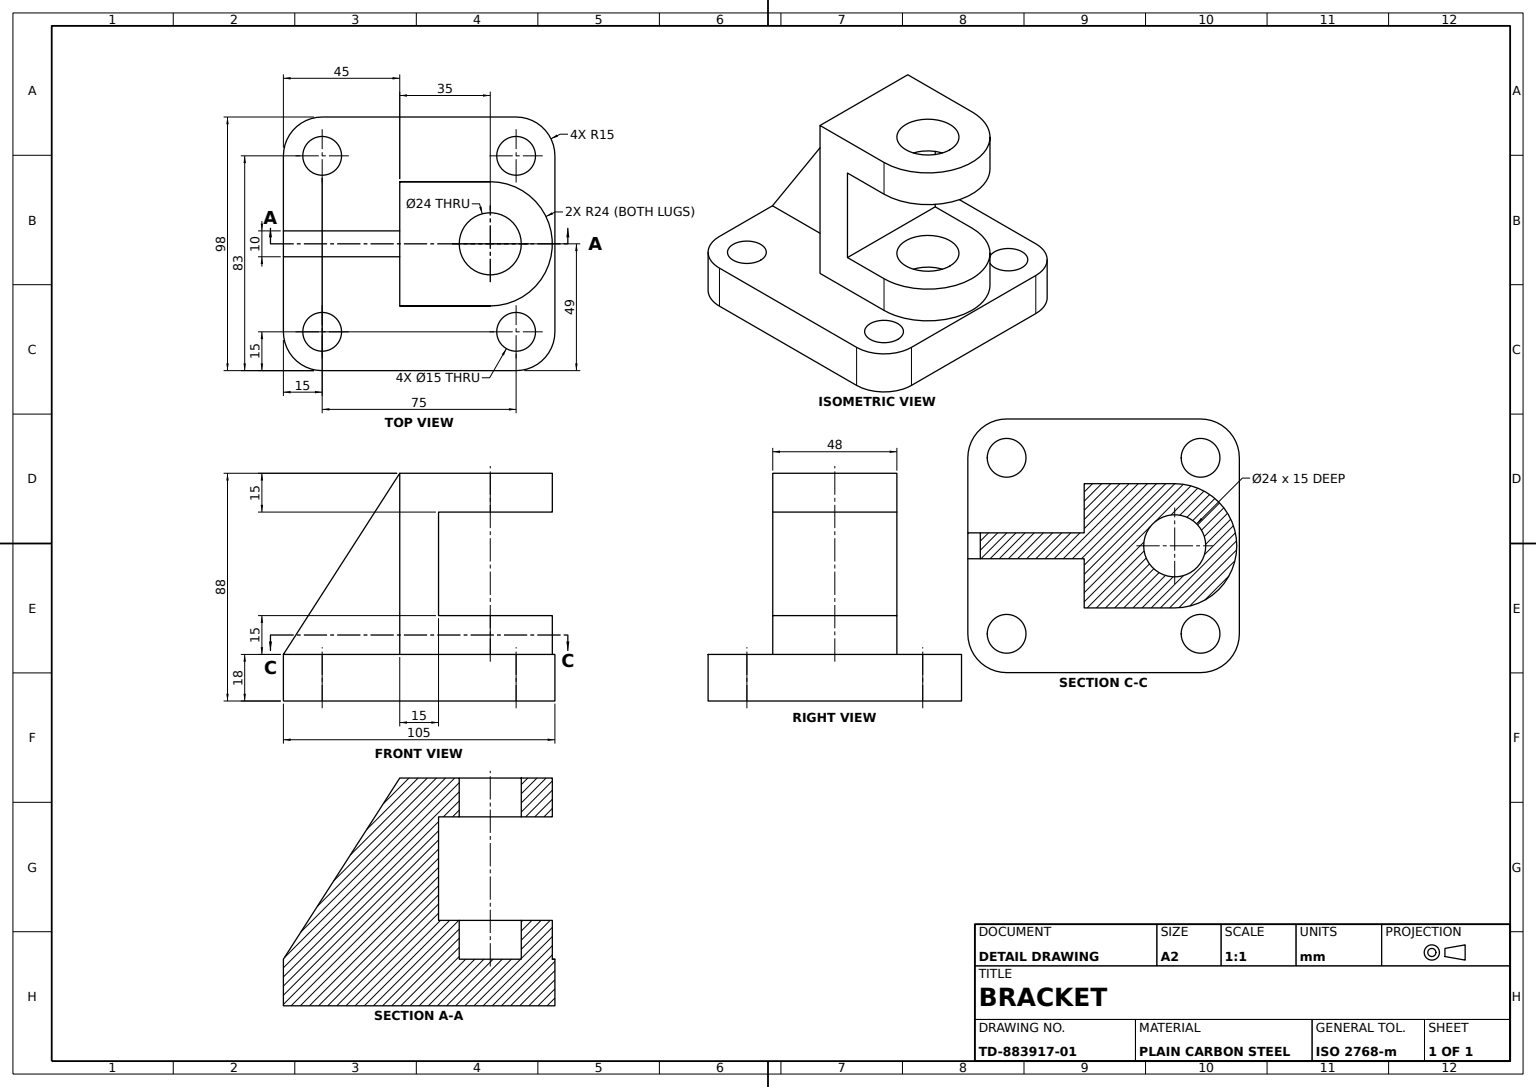
from build123d import *

# Parameters (mm, degrees)
BASE_PLATE_DEPTH           = 18
MOUNTING_HOLES_SKETCH_R    = 7.5
MOUNTING_HOLES_4X_15_DEPTH = 18
UPRIGHT_COLUMN_SKETCH_W    = 48
UPRIGHT_COLUMN_SKETCH_H    = 70
UPRIGHT_COLUMN_DEPTH       = 7.5
SUPPORT_RIB_REACH          = 115.584
SUPPORT_RIB_SKETCH_WALL_W  = 312.383924088
SUPPORT_RIB_SKETCH_WALL_H  = 10
CLEVIS_LUG_1_SKETCH_R      = 12
CLEVIS_LUG_1_DEPTH         = 15
CLEVIS_START               = 15
CLEVIS_LUG_2_SKETCH_R      = 12
CLEVIS_LUG_2_DEPTH         = 15


with BuildPart() as part:
    # Base Plate Sketch → Base Plate (new body)
    with BuildSketch(Plane(origin=(0, 0, 0), x_dir=(1, 0, 0), z_dir=(0, 1, 0))):
        with BuildLine():
            Line((-34, -52.5), (34, -52.5))
            ThreePointArc((34, -52.5), (44.606601718, -48.106601718), (49, -37.5))
            Line((49, -37.5), (49, 37.5))
            ThreePointArc((49, 37.5), (44.606601718, 48.106601718), (34, 52.5))
            Line((34, 52.5), (-34, 52.5))
            ThreePointArc((-34, 52.5), (-44.606601718, 48.106601718), (-49, 37.5))
            Line((-49, 37.5), (-49, -37.5))
            ThreePointArc((-49, -37.5), (-44.606601718, -48.106601718), (-34, -52.5))
        make_face()
    extrude(amount=BASE_PLATE_DEPTH)

    # Mounting Holes Sketch → Mounting Holes 4xØ15 (cut)
    with BuildSketch(Plane(origin=(0, 18, 0), x_dir=(1, 0, 0), z_dir=(0, 1, 0))):
        with Locations(Location((-34, 37.5, 0), (0, 0, 270))):
            Circle(MOUNTING_HOLES_SKETCH_R)
        with Locations(Location((34, 37.5, 0), (0, 0, 270))):
            Circle(MOUNTING_HOLES_SKETCH_R)
        with Locations(Location((-34, -37.5, 0), (0, 0, 270))):
            Circle(MOUNTING_HOLES_SKETCH_R)
        with Locations(Location((34, -37.5, 0), (0, 0, 270))):
            Circle(MOUNTING_HOLES_SKETCH_R)
    extrude(amount=-MOUNTING_HOLES_4X_15_DEPTH, mode=Mode.SUBTRACT)

    # Upright Column Sketch → Upright Column (add, symmetric)
    with BuildSketch(Plane.XY):
        with Locations((0, 53)):
            Rectangle(UPRIGHT_COLUMN_SKETCH_W, UPRIGHT_COLUMN_SKETCH_H)
    extrude(amount=UPRIGHT_COLUMN_DEPTH, both=True)

    # Support Rib Sketch wall → Support Rib (add, up to next)
    with BuildSketch(Plane(origin=(0, 53, 30), x_dir=(0, -0.841178475377, 0.540757591313), z_dir=(0, -0.540757591313, -0.841178475377)), mode=Mode.PRIVATE) as support_rib_sk1:
        Rectangle(SUPPORT_RIB_SKETCH_WALL_W, SUPPORT_RIB_SKETCH_WALL_H)
    support_rib_tool1 = extrude(support_rib_sk1.sketch, amount=SUPPORT_RIB_REACH, mode=Mode.PRIVATE) - part.part
    add(support_rib_tool1.solids().sort_by_distance((0, 53, 30))[0])

    # Clevis Lug 1 Sketch → Clevis Lug 1 (add)
    with BuildSketch(Plane(origin=(0, 88, 0), x_dir=(1, 0, 0), z_dir=(0, 1, 0))):
        with BuildLine():
            Line((-24, -7.5), (-24, 27.5))
            ThreePointArc((-24, 27.5), (0, 51.5), (24, 27.5))
            Line((24, 27.5), (24, -7.5))
            Line((24, -7.5), (-24, -7.5))
        make_face()
        with Locations(Location((0, 27.5, 0), (0, 0, 270))):
            Circle(CLEVIS_LUG_1_SKETCH_R, mode=Mode.SUBTRACT)
    extrude(amount=-CLEVIS_LUG_1_DEPTH)

    # Clevis Lug 2 Sketch → Clevis Lug 2 (add)
    with BuildSketch(Plane(origin=(0, 18, 0), x_dir=(1, 0, 0), z_dir=(0, 1, 0)).offset(CLEVIS_START)):
        with BuildLine():
            Line((-24, 27.5), (-24, 7.5))
            Line((-24, 7.5), (24, 7.5))
            Line((24, 7.5), (24, 27.5))
            ThreePointArc((24, 27.5), (0, 51.5), (-24, 27.5))
        make_face()
        with Locations(Location((0, 27.5, 0), (0, 0, 270))):
            Circle(CLEVIS_LUG_2_SKETCH_R, mode=Mode.SUBTRACT)
    extrude(amount=-CLEVIS_LUG_2_DEPTH)


solid = part.part
